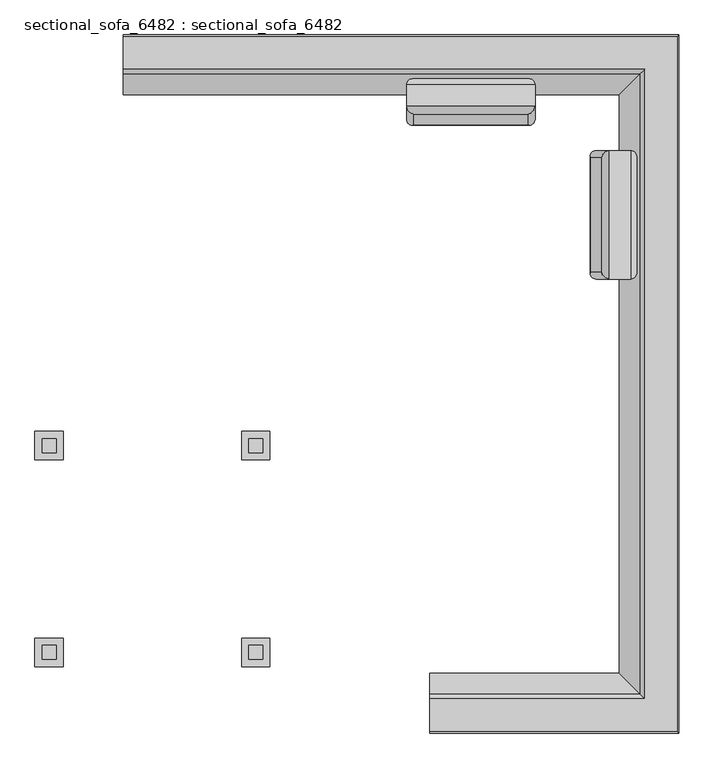
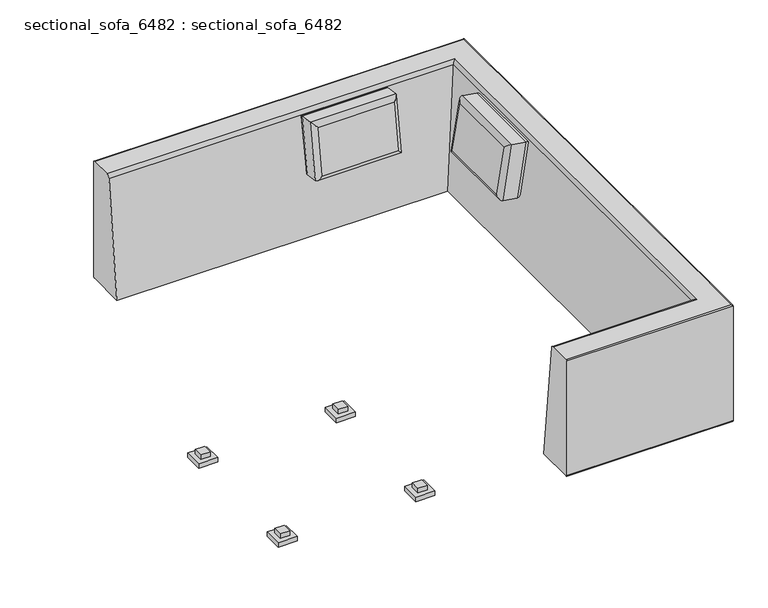
"""IFC4 building model written with IfcOpenShell, lengths in millimetres: proxy geometry, sectional_sofa_6482 : sectional_sofa_6482."""

from ifc_helpers import new_model, si_unit, frame, origin, place, context, project, spatial, circle_curve, ellipse_curve, faceted_brep, source, transform, mapped, element, save
from ifc_brep_helpers import plane_surface, cylinder_surface, advanced_brep


def sectional_sofa_6482_sectional_sofa_6482_9496661e(model_context):
    return source(origin(), model_context, "Body", "SolidModel", [
        advanced_brep(
        [(-712.932438, 1291.6931081, 704.85), (-712.932438, 1291.6931081, 57.15), (-712.932438, 1285.3431081, 50.8), (-712.932438, 1078.6460027, 50.8), (-712.932438, 1150.9219827, 695.9470238), (-712.932438, 1169.5897386, 711.2), (-712.932438, 1285.3431081, 711.2), (1268.267562, 1291.6931081, 704.85), (1268.267562, 1291.6931081, 57.15), (1261.917562, 1285.3431081, 50.8), (1261.917562, -1191.1568919, 50.8), (379.267562, -1191.1568919, 50.8), (379.267562, -984.4597865, 50.8), (1055.2204567, -984.4597865, 50.8), (1055.2204567, 1078.6460027, 50.8), (1127.4964367, 1150.9219827, 695.9470238), (1146.1641926, 1169.5897386, 711.2), (1146.1641926, -1075.4035225, 711.2), (379.267562, -1075.4035225, 711.2), (379.267562, -1191.1568919, 711.2), (1261.917562, -1191.1568919, 711.2), (1261.917562, 1285.3431081, 711.2), (1268.267562, -1197.5068919, 704.85), (1268.267562, -1197.5068919, 57.15), (1127.4964367, -1056.7357665, 695.9470238), (379.267562, -1197.5068919, 57.15), (379.267562, -1197.5068919, 704.85), (379.267562, -1056.7357665, 695.9470238)],
        [
            (0, 1),
            (1, 2, circle_curve(frame((-712.932438, 1285.3431081, 57.15), z_axis=(-1.0, 0.0, 0.0), x_axis=(0.0, -1.0, 0.0)), 6.35)),
            (2, 3),
            (3, 4, circle_curve(frame((-712.932438, 4725.645818, -31.1522279), z_axis=(-1.0, 0.0, 0.0), x_axis=(0.0, -1.0, 0.0)), 3647.9204789)),
            (4, 5, circle_curve(frame((-712.932438, 1169.5897386, 692.15), z_axis=(-1.0, 0.0, 0.0), x_axis=(0.0, -1.0, 0.0)), 19.05)),
            (5, 6),
            (6, 0, circle_curve(frame((-712.932438, 1285.3431081, 704.85), z_axis=(-1.0, 0.0, 0.0), x_axis=(0.0, -1.0, 0.0)), 6.35)),
            (0, 7),
            (7, 8),
            (8, 1),
            (8, 9, ellipse_curve(frame((1261.917562, 1285.3431081, 57.15), z_axis=(-0.7071067811865475, 0.7071067811865475, 0.0), x_axis=(-0.7071067811865476, -0.7071067811865474, 0.0)), 8.9802561, 6.35)),
            (9, 2),
            (9, 10),
            (10, 11),
            (11, 12),
            (12, 13),
            (13, 14),
            (14, 3),
            (14, 15, ellipse_curve(frame((4702.2202719, 4725.645818, -31.1522279), z_axis=(-0.7071067811865475, 0.7071067811865475, 0.0), x_axis=(-0.7071067811865476, -0.7071067811865474, 0.0)), 5158.9386157, 3647.9204789)),
            (15, 4),
            (15, 16, ellipse_curve(frame((1146.1641926, 1169.5897386, 692.15), z_axis=(-0.7071067811865475, 0.7071067811865475, 0.0), x_axis=(-0.7071067811865476, -0.7071067811865474, 0.0)), 26.9407684, 19.05)),
            (16, 5),
            (16, 17),
            (17, 18),
            (18, 19),
            (19, 20),
            (20, 21),
            (21, 6),
            (21, 7, ellipse_curve(frame((1261.917562, 1285.3431081, 704.85), z_axis=(-0.7071067811865475, 0.7071067811865475, 0.0), x_axis=(-0.7071067811865476, -0.7071067811865474, 0.0)), 8.9802561, 6.35)),
            (7, 22),
            (22, 23),
            (23, 8),
            (23, 10, ellipse_curve(frame((1261.917562, -1191.1568919, 57.15), z_axis=(0.7071067811865475, 0.7071067811865475, 0.0), x_axis=(-0.7071067811865474, 0.7071067811865476, 0.0)), 8.9802561, 6.35)),
            (13, 24, ellipse_curve(frame((4702.2202719, -4631.4596018, -31.1522279), z_axis=(0.7071067811865475, 0.7071067811865475, 0.0), x_axis=(-0.7071067811865474, 0.7071067811865476, 0.0)), 5158.9386157, 3647.9204789)),
            (24, 15),
            (24, 17, ellipse_curve(frame((1146.1641926, -1075.4035225, 692.15), z_axis=(0.7071067811865475, 0.7071067811865475, 0.0), x_axis=(-0.7071067811865474, 0.7071067811865476, 0.0)), 26.9407684, 19.05)),
            (20, 22, ellipse_curve(frame((1261.917562, -1191.1568919, 704.85), z_axis=(0.7071067811865475, 0.7071067811865475, 0.0), x_axis=(-0.7071067811865474, 0.7071067811865476, 0.0)), 8.9802561, 6.35)),
            (11, 25, circle_curve(frame((379.267562, -1191.1568919, 57.15), z_axis=(-1.0, 0.0, 0.0), x_axis=(0.0, 1.0, 0.0)), 6.35)),
            (25, 26),
            (26, 19, circle_curve(frame((379.267562, -1191.1568919, 704.85), z_axis=(-1.0, 0.0, 0.0), x_axis=(0.0, 1.0, 0.0)), 6.35)),
            (18, 27, circle_curve(frame((379.267562, -1075.4035225, 692.15), z_axis=(-1.0, 0.0, 0.0), x_axis=(0.0, 1.0, 0.0)), 19.05)),
            (27, 12, circle_curve(frame((379.267562, -4631.4596018, -31.1522279), z_axis=(-1.0, 0.0, 0.0), x_axis=(0.0, 1.0, 0.0)), 3647.9204789)),
            (22, 26),
            (25, 23),
            (27, 24),
        ],
        [
            plane_surface(frame((-712.932438, 1291.6931081, 50.8), z_axis=(-1.0, 0.0, 0.0), x_axis=(0.0, 0.0, -1.0))),
            plane_surface(frame((-712.932438, 1291.6931081, 704.85), z_axis=(0.0, 1.0, 0.0), x_axis=(1.0, 0.0, 0.0))),
            cylinder_surface(frame((-712.932438, 1285.3431081, 57.15), z_axis=(-1.0, 0.0, 0.0), x_axis=(0.0, -1.0, 0.0)), 6.35),
            plane_surface(frame((-712.932438, 1285.3431081, 50.8), z_axis=(0.0, 0.0, -1.0), x_axis=(1.0, 0.0, 0.0))),
            cylinder_surface(frame((-712.932438, 4725.645818, -31.1522279), z_axis=(-1.0, 0.0, 0.0), x_axis=(0.0, -1.0, 0.0)), 3647.9204789),
            cylinder_surface(frame((-712.932438, 1169.5897386, 692.15), z_axis=(-1.0, 0.0, 0.0), x_axis=(0.0, -1.0, 0.0)), 19.05),
            plane_surface(frame((-712.932438, 1169.5897386, 711.2), z_axis=(0.0, 0.0, 1.0), x_axis=(1.0, 0.0, 0.0))),
            cylinder_surface(frame((-712.932438, 1285.3431081, 704.85), z_axis=(-1.0, 0.0, 0.0), x_axis=(0.0, -1.0, 0.0)), 6.35),
            plane_surface(frame((1268.267562, 1291.6931081, 704.85), z_axis=(1.0, 0.0, 0.0), x_axis=(0.0, -1.0, 0.0))),
            cylinder_surface(frame((1261.917562, 1291.6931081, 57.15), z_axis=(0.0, 1.0, 0.0), x_axis=(-1.0, 0.0, 0.0)), 6.35),
            cylinder_surface(frame((4702.2202719, 1291.6931081, -31.1522279), z_axis=(0.0, 1.0, 0.0), x_axis=(-1.0, 0.0, 0.0)), 3647.9204789),
            cylinder_surface(frame((1146.1641926, 1291.6931081, 692.15), z_axis=(0.0, 1.0, 0.0), x_axis=(-1.0, 0.0, 0.0)), 19.05),
            cylinder_surface(frame((1261.917562, 1291.6931081, 704.85), z_axis=(0.0, 1.0, 0.0), x_axis=(-1.0, 0.0, 0.0)), 6.35),
            plane_surface(frame((379.267562, -1197.5068919, 50.8), z_axis=(-1.0, 0.0, 0.0), x_axis=(0.0, 0.0, -1.0))),
            plane_surface(frame((1268.267562, -1197.5068919, 704.85), z_axis=(0.0, -1.0, 0.0), x_axis=(-1.0, 0.0, 0.0))),
            cylinder_surface(frame((1268.267562, -1191.1568919, 57.15), z_axis=(1.0, 0.0, 0.0), x_axis=(0.0, 1.0, 0.0)), 6.35),
            cylinder_surface(frame((1268.267562, -4631.4596018, -31.1522279), z_axis=(1.0, 0.0, 0.0), x_axis=(0.0, 1.0, 0.0)), 3647.9204789),
            cylinder_surface(frame((1268.267562, -1075.4035225, 692.15), z_axis=(1.0, 0.0, 0.0), x_axis=(0.0, 1.0, 0.0)), 19.05),
            cylinder_surface(frame((1268.267562, -1191.1568919, 704.85), z_axis=(1.0, 0.0, 0.0), x_axis=(0.0, 1.0, 0.0)), 6.35),
        ],
        [
            (0, [[1, 2, 3, 4, 5, 6, 7]]),
            (1, [[-1, 8, 9, 10]]),
            (2, [[-2, -10, 11, 12]]),
            (3, [[-3, -12, 13, 14, 15, 16, 17, 18]]),
            (4, [[-4, -18, 19, 20]]),
            (5, [[-5, -20, 21, 22]]),
            (6, [[-6, -22, 23, 24, 25, 26, 27, 28]]),
            (7, [[-7, -28, 29, -8]]),
            (8, [[-9, 30, 31, 32]]),
            (9, [[-11, -32, 33, -13]]),
            (10, [[-17, 34, 35, -19]]),
            (11, [[-21, -35, 36, -23]]),
            (12, [[-27, 37, -30, -29]]),
            (13, [[-15, 38, 39, 40, -25, 41, 42]]),
            (14, [[-31, 43, -39, 44]]),
            (15, [[-14, -33, -44, -38]]),
            (16, [[-16, -42, 45, -34]]),
            (17, [[-24, -36, -45, -41]]),
            (18, [[-26, -40, -43, -37]]),
        ],
    ),
        advanced_brep(
        [(754.9501866, 990.6789418, 428.302718), (754.9501866, 1065.9407934, 416.3824117), (754.9501866, 1113.6220183, 717.429818), (754.9501866, 1038.3601668, 729.3501242), (297.7501866, 1038.3601668, 729.3501242), (297.7501866, 1113.6220183, 717.429818), (297.7501866, 1065.9407934, 416.3824117), (297.7501866, 990.6789418, 428.302718), (323.1501866, 1095.0015126, 437.4962602), (323.1501866, 1134.7358668, 688.3690987), (729.5501866, 1134.7358668, 688.3690987), (729.5501866, 1095.0015126, 437.4962602), (323.1501866, 1009.2994475, 708.2362758), (323.1501866, 969.5650934, 457.3634372), (729.5501866, 969.5650934, 457.3634372), (729.5501866, 1009.2994475, 708.2362758)],
        [
            (0, 1),
            (1, 2),
            (2, 3),
            (3, 0),
            (4, 5),
            (5, 6),
            (6, 7),
            (7, 4),
            (0, 7),
            (6, 1),
            (8, 9),
            (9, 10),
            (10, 11),
            (11, 8),
            (2, 5),
            (4, 3),
            (12, 13),
            (13, 14),
            (14, 15),
            (15, 12),
            (7, 13, ellipse_curve(frame((323.1501866, 994.6523772, 453.3900018), z_axis=(-0.7071067811865474, 0.1106158710412283, 0.6984011233337117), x_axis=(-0.7071067811865474, -0.11061587104122816, -0.6984011233337117)), 35.9210245, 25.4)),
            (12, 4, ellipse_curve(frame((323.1501866, 1034.3867314, 704.2628403), z_axis=(-0.7071067811865476, -0.11061587104122826, -0.6984011233337116), x_axis=(0.7071067811865475, -0.11061587104122819, -0.6984011233337117)), 35.9210245, 25.4)),
            (8, 6, ellipse_curve(frame((323.1501866, 1069.9142288, 441.4696956), z_axis=(-0.7071067811865474, 0.11061587104122826, 0.6984011233337117), x_axis=(-0.7071067811865474, -0.11061587104122816, -0.6984011233337117)), 35.9210245, 25.4)),
            (5, 9, ellipse_curve(frame((323.1501866, 1109.6485829, 692.3425341), z_axis=(-0.7071067811865476, -0.11061587104122823, -0.6984011233337116), x_axis=(0.7071067811865475, -0.11061587104122819, -0.6984011233337117)), 35.9210245, 25.4)),
            (0, 14, ellipse_curve(frame((729.5501866, 994.6523772, 453.3900018), z_axis=(-0.7071067811865476, -0.11061587104122807, -0.6984011233337117), x_axis=(0.7071067811865475, -0.11061587104122819, -0.6984011233337117)), 35.9210245, 25.4)),
            (11, 1, ellipse_curve(frame((729.5501866, 1069.9142288, 441.4696956), z_axis=(-0.7071067811865476, -0.11061587104122811, -0.6984011233337117), x_axis=(0.7071067811865475, -0.11061587104122819, -0.6984011233337117)), 35.9210245, 25.4)),
            (3, 15, ellipse_curve(frame((729.5501866, 1034.3867314, 704.2628403), z_axis=(0.7071067811865475, -0.1106158710412281, -0.6984011233337117), x_axis=(0.7071067811865474, 0.11061587104122819, 0.6984011233337117)), 35.9210245, 25.4)),
            (10, 2, ellipse_curve(frame((729.5501866, 1109.6485829, 692.3425341), z_axis=(0.7071067811865474, -0.11061587104122812, -0.6984011233337117), x_axis=(0.7071067811865475, 0.1106158710412282, 0.6984011233337118)), 35.9210245, 25.4)),
        ],
        [
            plane_surface(frame((754.9501866, 1077.8583572, 254.0), z_axis=(1.0, 0.0, 0.0), x_axis=(0.0, 0.0, 1.0))),
            plane_surface(frame((297.7501866, 1077.8583572, 254.0), z_axis=(-1.0, 0.0, 0.0), x_axis=(0.0, 0.0, 1.0))),
            plane_surface(frame((754.9501866, 965.591658, 432.2761534), z_axis=(0.0, -0.15643446504021818, -0.9876883405951399), x_axis=(-1.0, 0.0, 0.0))),
            plane_surface(frame((754.9501866, 1091.0280772, 412.4089763), z_axis=(0.0, 0.9876883405951399, -0.15643446504021818), x_axis=(-1.0, 0.0, 0.0))),
            plane_surface(frame((754.9501866, 1138.7093022, 713.4563825), z_axis=(0.0, 0.15643446504021818, 0.9876883405951399), x_axis=(-1.0, 0.0, 0.0))),
            plane_surface(frame((754.9501866, 1013.2728829, 733.3235596), z_axis=(0.0, -0.9876883405951399, 0.15643446504021818), x_axis=(-1.0, 0.0, 0.0))),
            cylinder_surface(frame((323.1501866, 1038.3601668, 729.3501242), z_axis=(0.0, -0.15643446504021827, -0.9876883405951398), x_axis=(1.0, 0.0, 0.0)), 25.4),
            cylinder_surface(frame((323.1501866, 1113.6220183, 717.429818), z_axis=(0.0, -0.15643446504021824, -0.9876883405951398), x_axis=(1.0, 0.0, 0.0)), 25.4),
            cylinder_surface(frame((297.7501866, 994.6523772, 453.3900018), z_axis=(1.0, 0.0, 0.0), x_axis=(0.0, 0.15643446504021824, 0.9876883405951398)), 25.4),
            cylinder_surface(frame((297.7501866, 1069.9142288, 441.4696956), z_axis=(1.0, 0.0, 0.0), x_axis=(0.0, 0.15643446504021957, 0.9876883405951395)), 25.4),
            cylinder_surface(frame((729.5501866, 990.6789418, 428.302718), z_axis=(0.0, 0.15643446504021813, 0.9876883405951398), x_axis=(-1.0, 0.0, 0.0)), 25.4),
            cylinder_surface(frame((729.5501866, 1065.9407934, 416.3824117), z_axis=(0.0, 0.15643446504021816, 0.9876883405951398), x_axis=(-1.0, 0.0, 0.0)), 25.4),
            cylinder_surface(frame((754.9501866, 1034.3867314, 704.2628403), z_axis=(-1.0, 0.0, 0.0), x_axis=(0.0, -0.15643446504021813, -0.9876883405951398)), 25.4),
            cylinder_surface(frame((754.9501866, 1109.6485829, 692.3425341), z_axis=(-1.0, 0.0, 0.0), x_axis=(0.0, -0.1564344650402168, -0.98768834059514)), 25.4),
        ],
        [
            (0, [[1, 2, 3, 4]]),
            (1, [[5, 6, 7, 8]]),
            (2, [[-1, 9, -7, 10]]),
            (3, [[11, 12, 13, 14]]),
            (4, [[-3, 15, -5, 16]]),
            (5, [[17, 18, 19, 20]]),
            (6, [[21, -17, 22, -8]]),
            (7, [[23, -6, 24, -11]]),
            (8, [[-21, -9, 25, -18]]),
            (9, [[-23, -14, 26, -10]]),
            (10, [[-25, -4, 27, -19]]),
            (11, [[-26, -13, 28, -2]]),
            (12, [[-22, -20, -27, -16]]),
            (13, [[-24, -15, -28, -12]]),
        ],
    ),
        advanced_brep(
        [(972.5408994, 421.3757369, 422.7530414), (1047.802751, 421.3757369, 410.8327352), (1095.4839759, 421.3757369, 711.8801414), (1020.2221244, 421.3757369, 723.8004476), (1020.2221244, 878.5757369, 723.8004476), (1095.4839759, 878.5757369, 711.8801414), (1047.802751, 878.5757369, 410.8327352), (972.5408994, 878.5757369, 422.7530414), (1076.8634702, 853.1757369, 431.9465836), (1116.5978244, 853.1757369, 682.8194221), (1116.5978244, 446.7757369, 682.8194221), (1076.8634702, 446.7757369, 431.9465836), (991.1614051, 853.1757369, 702.6865992), (951.427051, 853.1757369, 451.8137607), (951.427051, 446.7757369, 451.8137607), (991.1614051, 446.7757369, 702.6865992)],
        [
            (0, 1),
            (1, 2),
            (2, 3),
            (3, 0),
            (4, 5),
            (5, 6),
            (6, 7),
            (7, 4),
            (0, 7),
            (6, 1),
            (8, 9),
            (9, 10),
            (10, 11),
            (11, 8),
            (2, 5),
            (4, 3),
            (12, 13),
            (13, 14),
            (14, 15),
            (15, 12),
            (7, 13, ellipse_curve(frame((976.5143348, 853.1757369, 447.8403253), z_axis=(0.11061587104122693, 0.7071067811865475, 0.698401123333712), x_axis=(-0.11061587104122939, 0.7071067811865475, -0.6984011233337115)), 35.9210245, 25.4)),
            (12, 4, ellipse_curve(frame((1016.248689, 853.1757369, 698.7131638), z_axis=(-0.11061587104122933, 0.7071067811865474, -0.6984011233337116), x_axis=(-0.11061587104122698, -0.7071067811865476, -0.6984011233337118)), 35.9210245, 25.4)),
            (8, 6, ellipse_curve(frame((1051.7761864, 853.1757369, 435.920019), z_axis=(0.11061587104122693, 0.7071067811865475, 0.698401123333712), x_axis=(-0.11061587104122939, 0.7071067811865475, -0.6984011233337115)), 35.9210245, 25.4)),
            (5, 9, ellipse_curve(frame((1091.5105405, 853.1757369, 686.7928575), z_axis=(-0.11061587104122934, 0.7071067811865474, -0.6984011233337116), x_axis=(-0.11061587104122697, -0.7071067811865476, -0.6984011233337118)), 35.9210245, 25.4)),
            (0, 14, ellipse_curve(frame((976.5143348, 446.7757369, 447.8403253), z_axis=(-0.11061587104122948, 0.7071067811865474, -0.6984011233337116), x_axis=(-0.11061587104122696, -0.7071067811865478, -0.6984011233337116)), 35.9210245, 25.4)),
            (11, 1, ellipse_curve(frame((1051.7761864, 446.7757369, 435.920019), z_axis=(-0.11061587104122947, 0.7071067811865474, -0.6984011233337116), x_axis=(-0.11061587104122693, -0.7071067811865478, -0.6984011233337116)), 35.9210245, 25.4)),
            (3, 15, ellipse_curve(frame((1016.248689, 446.7757369, 698.7131638), z_axis=(-0.11061587104122703, -0.7071067811865477, -0.6984011233337116), x_axis=(0.11061587104122943, -0.7071067811865472, 0.6984011233337117)), 35.9210245, 25.4)),
            (10, 2, ellipse_curve(frame((1091.5105405, 446.7757369, 686.7928575), z_axis=(-0.11061587104122698, -0.7071067811865477, -0.6984011233337116), x_axis=(0.11061587104122943, -0.7071067811865472, 0.6984011233337117)), 35.9210245, 25.4)),
        ],
        [
            plane_surface(frame((1059.7203148, 421.3757369, 248.4503234), z_axis=(0.0, -1.0, 0.0), x_axis=(0.0, 0.0, 1.0))),
            plane_surface(frame((1059.7203148, 878.5757369, 248.4503234), z_axis=(0.0, 1.0, 0.0), x_axis=(0.0, 0.0, 1.0))),
            plane_surface(frame((947.4536156, 421.3757369, 426.7264768), z_axis=(-0.15643446504021818, 0.0, -0.9876883405951399), x_axis=(0.0, 1.0, 0.0))),
            plane_surface(frame((1072.8900348, 421.3757369, 406.8592998), z_axis=(0.9876883405951399, 0.0, -0.15643446504021818), x_axis=(0.0, 1.0, 0.0))),
            plane_surface(frame((1120.5712598, 421.3757369, 707.906706), z_axis=(0.15643446504021818, 0.0, 0.9876883405951399), x_axis=(0.0, 1.0, 0.0))),
            plane_surface(frame((995.1348405, 421.3757369, 727.773883), z_axis=(-0.9876883405951399, 0.0, 0.15643446504021818), x_axis=(0.0, 1.0, 0.0))),
            cylinder_surface(frame((1020.2221244, 853.1757369, 723.8004476), z_axis=(-0.15643446504021816, 0.0, -0.9876883405951398), x_axis=(0.0, -1.0, 0.0)), 25.4),
            cylinder_surface(frame((1095.4839759, 853.1757369, 711.8801414), z_axis=(-0.15643446504021816, 0.0, -0.9876883405951398), x_axis=(0.0, -1.0, 0.0)), 25.4),
            cylinder_surface(frame((976.5143348, 878.5757369, 447.8403253), z_axis=(0.0, -1.0000000000000002, 0.0), x_axis=(0.15643446504021824, 0.0, 0.9876883405951399)), 25.4),
            cylinder_surface(frame((1051.7761864, 878.5757369, 435.920019), z_axis=(0.0, -1.0000000000000002, 0.0), x_axis=(0.15643446504022113, 0.0, 0.9876883405951394)), 25.4),
            cylinder_surface(frame((972.5408994, 446.7757369, 422.7530414), z_axis=(0.15643446504021827, 0.0, 0.9876883405951398), x_axis=(0.0, 1.0, 0.0)), 25.4),
            cylinder_surface(frame((1047.802751, 446.7757369, 410.8327352), z_axis=(0.15643446504021824, 0.0, 0.9876883405951398), x_axis=(0.0, 1.0, 0.0)), 25.4),
            cylinder_surface(frame((1016.248689, 421.3757369, 698.7131638), z_axis=(0.0, 1.0000000000000002, 0.0), x_axis=(-0.15643446504021816, 0.0, -0.9876883405951399)), 25.4),
            cylinder_surface(frame((1091.5105405, 421.3757369, 686.7928575), z_axis=(0.0, 1.0000000000000002, 0.0), x_axis=(-0.1564344650402153, 0.0, -0.9876883405951403)), 25.4),
        ],
        [
            (0, [[1, 2, 3, 4]]),
            (1, [[5, 6, 7, 8]]),
            (2, [[-1, 9, -7, 10]]),
            (3, [[11, 12, 13, 14]]),
            (4, [[-3, 15, -5, 16]]),
            (5, [[17, 18, 19, 20]]),
            (6, [[21, -17, 22, -8]]),
            (7, [[23, -6, 24, -11]]),
            (8, [[-21, -9, 25, -18]]),
            (9, [[-23, -14, 26, -10]]),
            (10, [[-25, -4, 27, -19]]),
            (11, [[-26, -13, 28, -2]]),
            (12, [[-22, -20, -27, -16]]),
            (13, [[-24, -15, -28, -12]]),
        ],
    ),
        faceted_brep([(-926.5924005, -223.6520518, 25.4), (-926.5924005, -122.0520518, 25.4), (-1028.1924005, -122.0520518, 25.4), (-1028.1924005, -223.6520518, 25.4), (-951.9924005, -147.4520518, 25.4), (-951.9924005, -198.2520518, 25.4), (-1002.7924005, -198.2520518, 25.4), (-1002.7924005, -147.4520518, 25.4), (-926.5924005, -223.6520518, 0.0), (-1028.1924005, -223.6520518, 0.0), (-1028.1924005, -122.0520518, 0.0), (-926.5924005, -122.0520518, 0.0), (-951.9924005, -198.2520518, 50.8), (-951.9924005, -147.4520518, 50.8), (-1002.7924005, -147.4520518, 50.8), (-1002.7924005, -198.2520518, 50.8)], [[[0, 1, 2, 3], [4, 5, 6, 7]], [[8, 9, 10, 11]], [[1, 0, 8, 11]], [[2, 1, 11, 10]], [[3, 2, 10, 9]], [[0, 3, 9, 8]], [[12, 13, 14, 15]], [[13, 12, 5, 4]], [[14, 13, 4, 7]], [[15, 14, 7, 6]], [[12, 15, 6, 5]]]),
        faceted_brep([(-291.5924005, -223.6520518, 25.4), (-189.9924005, -223.6520518, 25.4), (-189.9924005, -122.0520518, 25.4), (-291.5924005, -122.0520518, 25.4), (-215.3924005, -198.2520518, 25.4), (-266.1924005, -198.2520518, 25.4), (-266.1924005, -147.4520518, 25.4), (-215.3924005, -147.4520518, 25.4), (-291.5924005, -223.6520518, 0.0), (-291.5924005, -122.0520518, 0.0), (-189.9924005, -122.0520518, 0.0), (-189.9924005, -223.6520518, 0.0), (-266.1924005, -198.2520518, 50.8), (-215.3924005, -198.2520518, 50.8), (-215.3924005, -147.4520518, 50.8), (-266.1924005, -147.4520518, 50.8)], [[[0, 1, 2, 3], [4, 5, 6, 7]], [[8, 9, 10, 11]], [[1, 0, 8, 11]], [[2, 1, 11, 10]], [[3, 2, 10, 9]], [[0, 3, 9, 8]], [[12, 13, 14, 15]], [[13, 12, 5, 4]], [[14, 13, 4, 7]], [[15, 14, 7, 6]], [[12, 15, 6, 5]]]),
        faceted_brep([(-291.5924005, -960.2520518, 25.4), (-189.9924005, -960.2520518, 25.4), (-189.9924005, -858.6520518, 25.4), (-291.5924005, -858.6520518, 25.4), (-215.3924005, -934.8520518, 25.4), (-266.1924005, -934.8520518, 25.4), (-266.1924005, -884.0520518, 25.4), (-215.3924005, -884.0520518, 25.4), (-291.5924005, -960.2520518, 0.0), (-291.5924005, -858.6520518, 0.0), (-189.9924005, -858.6520518, 0.0), (-189.9924005, -960.2520518, 0.0), (-266.1924005, -934.8520518, 50.8), (-215.3924005, -934.8520518, 50.8), (-215.3924005, -884.0520518, 50.8), (-266.1924005, -884.0520518, 50.8)], [[[0, 1, 2, 3], [4, 5, 6, 7]], [[8, 9, 10, 11]], [[1, 0, 8, 11]], [[2, 1, 11, 10]], [[3, 2, 10, 9]], [[0, 3, 9, 8]], [[12, 13, 14, 15]], [[13, 12, 5, 4]], [[14, 13, 4, 7]], [[15, 14, 7, 6]], [[12, 15, 6, 5]]]),
        faceted_brep([(-926.5924005, -960.2520518, 25.4), (-926.5924005, -858.6520518, 25.4), (-1028.1924005, -858.6520518, 25.4), (-1028.1924005, -960.2520518, 25.4), (-951.9924005, -884.0520518, 25.4), (-951.9924005, -934.8520518, 25.4), (-1002.7924005, -934.8520518, 25.4), (-1002.7924005, -884.0520518, 25.4), (-926.5924005, -960.2520518, 0.0), (-1028.1924005, -960.2520518, 0.0), (-1028.1924005, -858.6520518, 0.0), (-926.5924005, -858.6520518, 0.0), (-951.9924005, -934.8520518, 50.8), (-951.9924005, -884.0520518, 50.8), (-1002.7924005, -884.0520518, 50.8), (-1002.7924005, -934.8520518, 50.8)], [[[0, 1, 2, 3], [4, 5, 6, 7]], [[8, 9, 10, 11]], [[1, 0, 8, 11]], [[2, 1, 11, 10]], [[3, 2, 10, 9]], [[0, 3, 9, 8]], [[12, 13, 14, 15]], [[13, 12, 5, 4]], [[14, 13, 4, 7]], [[15, 14, 7, 6]], [[12, 15, 6, 5]]]),
    ])


if __name__ == "__main__":
    model = new_model("IFC4")
    model_context = context("Model", 3, world=origin())
    ifc_project = project(units=[si_unit("LENGTHUNIT", "METRE", prefix="MILLI")], contexts=[model_context])
    site = spatial("IfcSite", under=ifc_project)
    building = spatial("IfcBuilding", under=site)
    placement = place(None, origin())
    sectional_sofa_6482_sectional_sofa_6482_shape = sectional_sofa_6482_sectional_sofa_6482_9496661e(model_context)
    element("IfcBuildingElementProxy", 1, Name="sectional_sofa_6482 : sectional_sofa_6482", ObjectType="sectional_sofa_6482 : sectional_sofa_6482", at=placement, inside=building, context=model_context, shape_type="MappedRepresentation", body=[
        mapped(sectional_sofa_6482_sectional_sofa_6482_shape, transform((0.0, 0.0, 0.0), x_axis=(1.0, 0.0, 0.0), y_axis=(0.0, 1.0, 0.0), z_axis=(0.0, 0.0, 1.0))),
    ])
    save(model, "model.ifc")

# Revit data of these elements
# Type "sectional_sofa_6482 : sectional_sofa_6482"
#   frame trim = frame trim
#   fabric = fabric
#   Frame = frame
#   FABRIC 2 = fabric 2
#   Default Elevation = 0
# Element 1 (IfcBuildingElementProxy, "sectional_sofa_6482 : sectional_sofa_6482")
#   Materials on its faces: "frame trim", "fabric", "fabric 2", "frame"
# Materials
#   "frame trim": class "Metal", colour RGB 182 182 182, transparency 0
#   "fabric": class "Leather", colour RGB 255 245 240, transparency 0
#   "frame": class "Wood", colour RGB 71 38 7, transparency 0
#   "fabric 2": class "Fabric", colour RGB 128 0 0, transparency 0
